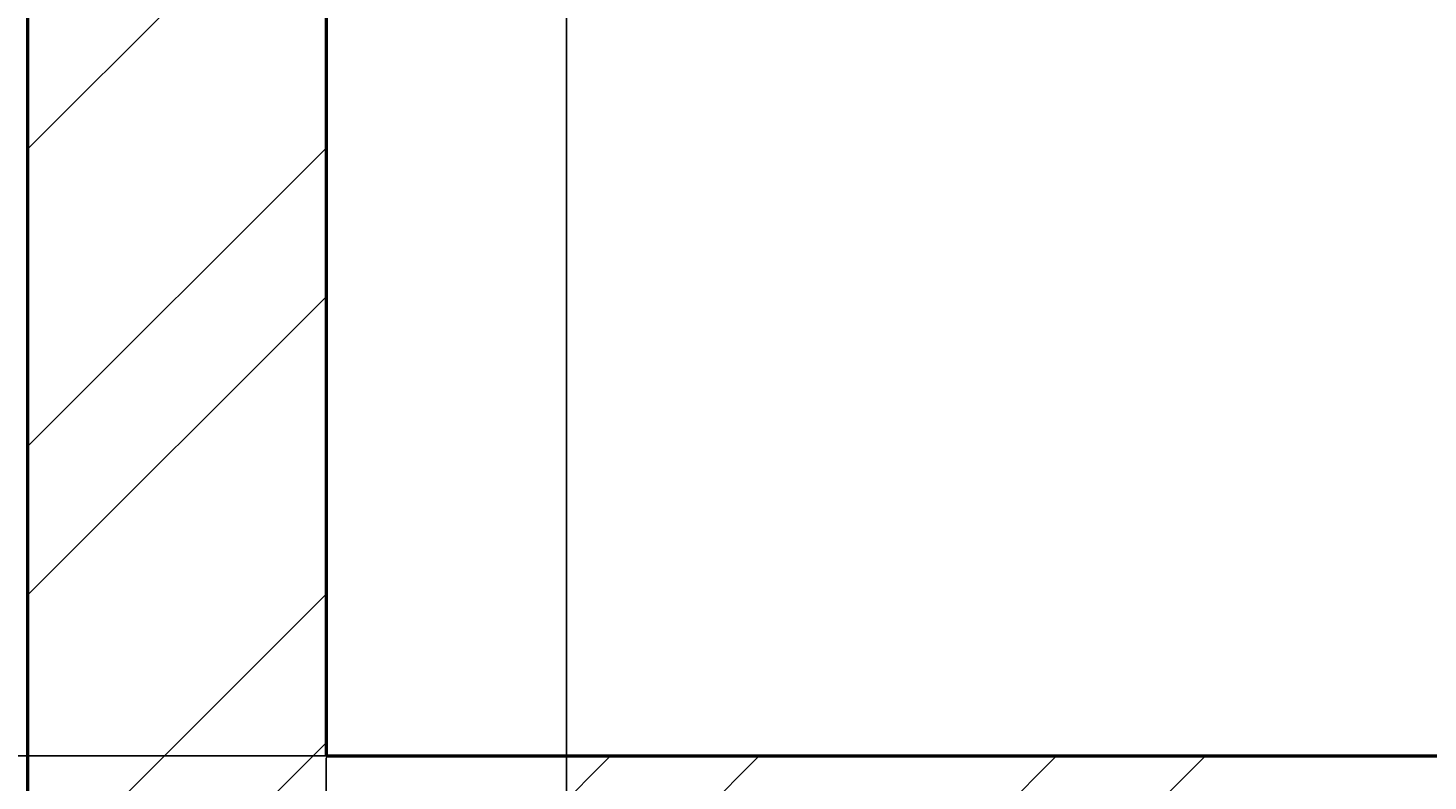
# Model space of a CAD drawing. Units: inches. Extents: x 2812 to 3051, y 1398 to 1659.
# Tile 46 of 65: x 2835 to 2878, y 1559 to 1582. Entities that reach past the tile are written whole.
import ezdxf

# ---------------------------------------------------------------- set-up
doc = ezdxf.new("R2010")
doc.units = ezdxf.units.IN
for name, color, linetype, lineweight in [('A-ANNO-DIMS', 2, 'Continuous', 18), ('S-CONC', 7, 'Continuous', 50), ('S-CONC-PATT', 8, 'Continuous', 18)]:
    doc.layers.add(name, color=color, linetype=linetype, lineweight=lineweight)
doc.styles.get("Standard").update_dxf_attribs({"font": 'arial.ttf'})
doc.dimstyles.get("Standard").update_dxf_attribs({"dimtxt": 0.18, "dimasz": 0.18, "dimexe": 0.18, "dimexo": 0.0625, "dimgap": 0.09, "dimtad": 0, "dimtih": 1, "dimtoh": 1, "dimdec": 4, "dimzin": 0, "dimdsep": 46, "dimtxsty": 'Standard', "dimcen": 0.09, "dimadec": 0, "dimazin": 0, "dimtfac": 1, "dimtdec": 4, "dimtofl": 0, "dimtmove": 0, "dimatfit": 3, "dimfxl": 1, "dimtolj": 1, "dimtzin": 0, "dimarcsym": 0})

# ---------------------------------------------------------------- blocks, each defined once
blk = doc.blocks.new('*D28')
at = {"layer": 'A-ANNO-DIMS', "color": 0, "lineweight": -2, "transparency": 16777216}
for p, q in [((2851.646, 1598.667), (2851.646, 1397.505)), ((2844.385, 1559.757), (2844.385, 1397.505)), ((2844.565, 1397.685), (2847.64, 1397.685)), ((2851.466, 1397.685), (2848.391, 1397.685))]:
    blk.add_line(p, q, dxfattribs=at)
at = {"layer": 'A-ANNO-DIMS', "color": 0, "transparency": 16777216}
for points in [[(2844.565, 1397.715), (2844.565, 1397.655), (2844.385, 1397.685)], [(2851.466, 1397.715), (2851.466, 1397.655), (2851.646, 1397.685)]]:
    blk.add_solid(points, dxfattribs=at)
at = {"layer": 'Defpoints', "color": 0, "transparency": 16777216}
for p in [(2851.646, 1598.73), (2844.385, 1559.82), (2851.646, 1397.685)]:
    blk.add_point(p, dxfattribs=at)
at = {"layer": 'A-ANNO-DIMS', "color": 0, "transparency": 16777216, "insert": (2848.016, 1397.685), "char_height": 0.18, "attachment_point": 5}
blk.add_mtext('\\A1;7.261', dxfattribs=at)
blk = doc.blocks.new('*D36')
at = {"layer": 'A-ANNO-DIMS', "color": 0, "lineweight": -2, "transparency": 16777216}
for p, q in [((2844.322, 1559.82), (2811.806, 1559.82)), ((2811.986, 1559.64), (2811.986, 1555.502)), ((2811.986, 1551), (2811.986, 1555.138)), ((2835.322, 1550.82), (2811.806, 1550.82))]:
    blk.add_line(p, q, dxfattribs=at)
at = {"layer": 'A-ANNO-DIMS', "color": 0, "transparency": 16777216}
for points in [[(2811.956, 1559.64), (2812.016, 1559.64), (2811.986, 1559.82)], [(2811.956, 1551), (2812.016, 1551), (2811.986, 1550.82)]]:
    blk.add_solid(points, dxfattribs=at)
at = {"layer": 'Defpoints', "color": 0, "transparency": 16777216}
for p in [(2811.986, 1559.82), (2844.385, 1559.82), (2835.385, 1550.82)]:
    blk.add_point(p, dxfattribs=at)
at = {"layer": 'A-ANNO-DIMS', "color": 0, "transparency": 16777216, "insert": (2811.986, 1555.32), "char_height": 0.18, "attachment_point": 5}
blk.add_mtext('\\A1;9', dxfattribs=at)
blk = doc.blocks.new('*D37')
at = {"layer": 'A-ANNO-DIMS', "color": 0, "lineweight": -2, "transparency": 16777216}
for p, q in [((2910.679, 1598.82), (2811.806, 1598.82)), ((2811.986, 1598.64), (2811.986, 1579.502)), ((2811.986, 1560), (2811.986, 1579.138)), ((2883.322, 1559.82), (2811.806, 1559.82))]:
    blk.add_line(p, q, dxfattribs=at)
at = {"layer": 'A-ANNO-DIMS', "color": 0, "transparency": 16777216}
for points in [[(2811.956, 1598.64), (2812.016, 1598.64), (2811.986, 1598.82)], [(2811.956, 1560), (2812.016, 1560), (2811.986, 1559.82)]]:
    blk.add_solid(points, dxfattribs=at)
at = {"layer": 'Defpoints', "color": 0, "transparency": 16777216}
for p in [(2811.986, 1598.82), (2910.742, 1598.82), (2883.385, 1559.82)]:
    blk.add_point(p, dxfattribs=at)
at = {"layer": 'A-ANNO-DIMS', "color": 0, "transparency": 16777216, "insert": (2811.986, 1579.32), "char_height": 0.18, "attachment_point": 5}
blk.add_mtext('\\A1;39', dxfattribs=at)

msp = doc.modelspace()

# ---------------------------------------------------------------- hatches: boundary and pattern name
at = {"layer": 'S-CONC-PATT'}
h = msp.add_hatch(dxfattribs=at)
h.set_pattern_fill('ANSI32', color=256)
h.paths.add_polyline_path([(3027.3849, 1646.82), (2835.3849, 1646.82), (2835.3849, 1603.2296), (2844.3849, 1603.2296), (2844.3849, 1637.82), (3018.3849, 1637.82), (3018.3849, 1602.5441), (3027.3849, 1602.5441)])
h.paths.add_polyline_path([(2844.3849, 1594.2296), (2835.3849, 1594.2296), (2835.3849, 1550.82), (3027.3849, 1550.82), (3027.3849, 1593.5441), (3018.3849, 1593.5441), (3018.3849, 1559.82), (2844.3849, 1559.82)])
h.paths.add_polyline_path([(2844.3849, 1482.0354), (2835.3849, 1482.0354), (2835.3849, 1463.4959), (2844.3849, 1463.4959)])
h.paths.add_polyline_path([(2844.3849, 1461.4959), (2835.3849, 1461.4959), (2835.3849, 1416.0354), (2844.3849, 1416.0354)])
h.paths.add_polyline_path([(3027.3849, 1482.0354), (3018.3849, 1482.0354), (3018.3849, 1463.2854), (3027.3849, 1463.2854)])
h.paths.add_polyline_path([(3027.3849, 1461.2854), (3018.3849, 1461.2854), (3018.3849, 1416.0354), (3027.3849, 1416.0354)])
h.paths.add_polyline_path([(2961.3849, 1448.4738), (2952.3849, 1448.4738), (2952.3849, 1416.0354), (2961.3849, 1416.0354)])
h.paths.add_polyline_path([(2961.3849, 1462.3026), (2952.3849, 1462.3026), (2952.3849, 1450.4738), (2961.3849, 1450.4738)])
h.paths.add_polyline_path([(2961.3849, 1472.0354), (2952.3849, 1472.0354), (2952.3849, 1462.3026), (2961.3849, 1462.3026)])

# ---------------------------------------------------------------- linework, layer by layer
at = {"layer": 'S-CONC'}
for p, q in [((2835.3849, 1550.82), (2835.3849, 1646.82)), ((2844.3849, 1637.82), (2844.3849, 1559.82)), ((2844.3849, 1559.82), (3018.3849, 1559.82))]:
    msp.add_line(p, q, dxfattribs=at)

# ---------------------------------------------------------------- dimensions: what is measured, and where the dimension line sits
at = {"layer": 'A-ANNO-DIMS'}
for base, p1, p2, picture, middle in [((2811.9855, 1598.82), (2883.3849, 1559.82), (2910.7415, 1598.82), '*D37', (2811.9855, 1579.32)), ((2811.9855, 1559.82), (2835.3849, 1550.82), (2844.3849, 1559.82), '*D36', (2811.9855, 1555.32))]:
    dim = msp.add_linear_dim(base=base, p1=p1, p2=p2, angle=90, dimstyle='Standard', override={"dimdec": 0, "dimlfac": 1, "dimrnd": 0, "dimzin": 0, "dimdsep": 46, "dimlunit": 2}, dxfattribs=at)
    dim.commit()
    dim.dimension.update_dxf_attribs({"geometry": picture, "text_midpoint": middle})
dim = msp.add_linear_dim(base=(2851.6462, 1397.6854), p1=(2844.3849, 1559.82), p2=(2851.6462, 1598.7296), dimstyle='Standard', override={"dimdec": 3, "dimlfac": 1, "dimrnd": 0, "dimzin": 0, "dimdsep": 46, "dimlunit": 2}, dxfattribs=at)
dim.commit()
dim.dimension.update_dxf_attribs({"geometry": '*D28', "text_midpoint": (2848.0156, 1397.6854)})

doc.saveas('drawing.dxf')
